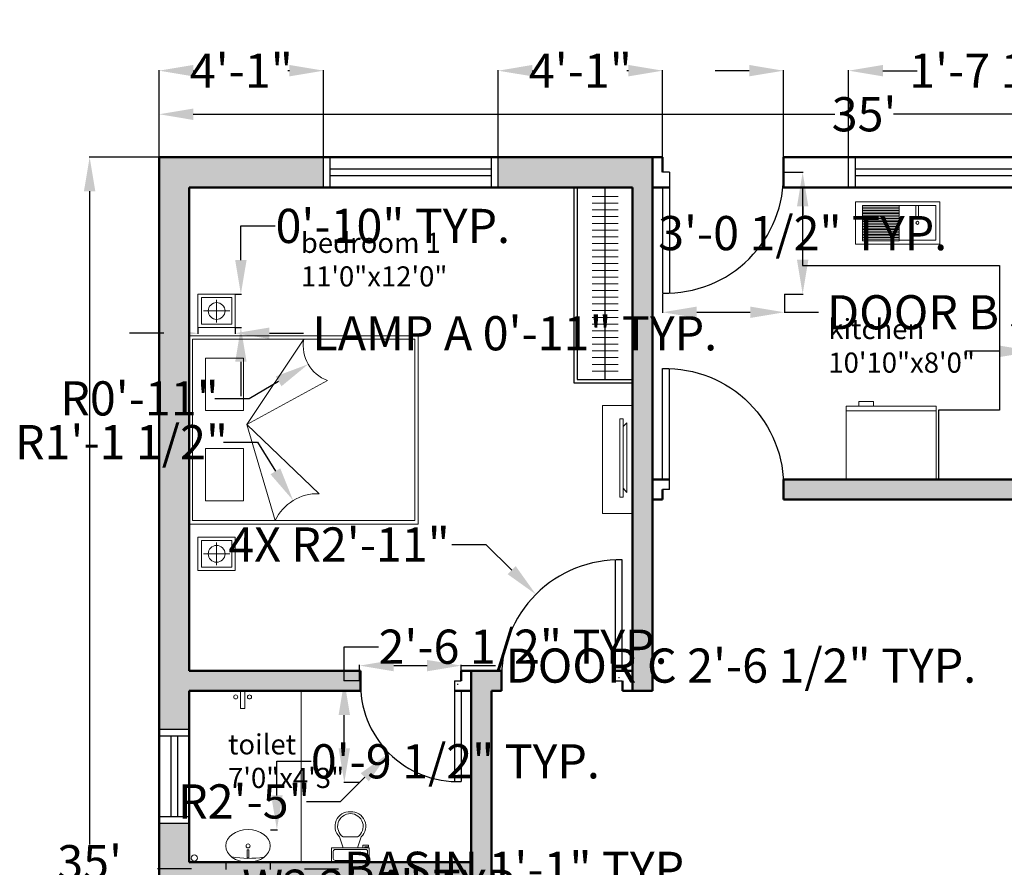
# Model space of a CAD drawing. Units: inches. Extents: x 18 to 9768, y 4 to 3529.
# Tile 2 of 6: x 8712 to 9006, y 3276 to 3529. Entities that reach past the tile are written whole.
import ezdxf

# ---------------------------------------------------------------- set-up
doc = ezdxf.new("R2010")
doc.units = ezdxf.units.IN
doc.header["$MEASUREMENT"] = 0
for name, color, linetype, lineweight in [('A-ANNO-DIMS', 2, 'Continuous', 18), ('A-AREA-IDEN', 7, 'Continuous', 18), ('A-CASE-PATT', 9, 'Continuous', 13), ('A-EQPM', 8, 'Continuous', 18), ('A-FLOR-CASE', 9, 'Continuous', 25), ('A-FLOR-FIXT', 9, 'Continuous', 18), ('A-FURN', 8, 'Continuous', 18), ('A-WALL-PATT', 252, 'Continuous', 13), ('WAL', 7, 'Continuous', 50)]:
    doc.layers.add(name, color=color, linetype=linetype, lineweight=lineweight)
doc.layers.add('A-DOOR', color=30, linetype='Continuous', lineweight=25, true_color=0xf8991e)
doc.layers.add('A-GLAZ', color=177, linetype='Continuous', lineweight=25, true_color=0x293189)
doc.styles.get("Standard").update_dxf_attribs({"font": 'arial.ttf'})
doc.dimstyles.get("Standard").update_dxf_attribs({"dimtxt": 10.18, "dimasz": 10.18, "dimexe": 0.18, "dimexo": 0.0625, "dimgap": 0.09, "dimtad": 0, "dimtih": 1, "dimtoh": 1, "dimdec": 0, "dimzin": 0, "dimdsep": 46, "dimlunit": 3, "dimtxsty": 'Standard', "dimcen": 0.09, "dimadec": 0, "dimazin": 0, "dimtfac": 1, "dimtdec": 0, "dimtofl": 0, "dimtmove": 0, "dimatfit": 3, "dimfxl": 1, "dimtolj": 1, "dimtzin": 0, "dimarcsym": 0})

# ---------------------------------------------------------------- blocks, each defined once
blk = doc.blocks.new('*U2')
for p, q in [((9.5, -6), (9.5, -2)), ((-10, -8.5), (-8, -8.5)), ((-10, -9.5), (-10, -8.5)), ((-7, -9.5), (-10, -9.5)), ((-8, -8.5), (-8, -8)), ((-7, -8), (-7, -9.5)), ((-4, -8), (-6, -14)), ((4, -8), (6, -14)), ((4, -14), (-4, -14))]:
    blk.add_line(p, q)
blk.add_lwpolyline([(10.5, -8), (10.5, 0), (-10.5, 0), (-10.5, -8)], close=True)
for points in [[(-9.5, -2), (-9.5, -6)], [(8.5, -1), (-8.5, -1)], [(-8.5, -7), (8.5, -7)]]:
    blk.add_lwpolyline(points)
for centre, radius, start, end in [((-8.625, -1.875), 0.8839, 81.8699, 188.1301), ((8.625, -1.875), 0.8839, 351.8699, 98.1301), ((-8.625, -6.125), 0.8839, 171.869898, 278.1301), ((8.625, -6.125), 0.8839, 261.8699, 8.1301), ((-0.4772, -19.9188), 8.0953, 133.01722, 273.38), ((0.0374, -19.8731), 7.127, 124.50543, 269.7), ((-0.0373, -19.8731), 7.127, 270.3, 55.4946), ((0.4773, -19.9188), 8.0953, 266.62, 46.9828)]:
    blk.add_arc(centre, radius, start, end)
blk = doc.blocks.new('*D3')
at = {"layer": 'A-ANNO-DIMS', "color": 0, "lineweight": -2, "transparency": 16777216}
for p, q in [((8753.89, 3487.8), (8753.89, 3500.68)), ((8764.07, 3500.5), (8955.16, 3500.5)), ((9163.71, 3500.5), (8972.61, 3500.5)), ((9173.89, 3487.8), (9173.89, 3500.68))]:
    blk.add_line(p, q, dxfattribs=at)
at = {"layer": 'A-ANNO-DIMS', "color": 0, "transparency": 16777216}
for points in [[(8764.07, 3502.19), (8764.07, 3498.8), (8753.89, 3500.5)], [(9163.71, 3502.19), (9163.71, 3498.8), (9173.89, 3500.5)]]:
    blk.add_solid(points, dxfattribs=at)
at = {"layer": 'Defpoints', "color": 0, "transparency": 16777216}
for p in [(9173.89, 3500.5), (8753.89, 3487.73), (9173.89, 3487.73)]:
    blk.add_point(p, dxfattribs=at)
at = {"layer": 'A-ANNO-DIMS', "color": 0, "transparency": 16777216, "insert": (8963.89, 3500.5), "char_height": 10.18, "attachment_point": 5}
blk.add_mtext("\\A1;35'", dxfattribs=at)
blk = doc.blocks.new('*D4')
at = {"layer": 'A-ANNO-DIMS', "color": 0, "lineweight": -2, "transparency": 16777216}
for p, q in [((8753.82, 3487.73), (8733.02, 3487.73)), ((8733.2, 3477.55), (8733.2, 3283.03)), ((8733.2, 3077.91), (8733.2, 3272.44)), ((8753.82, 3067.73), (8733.02, 3067.73))]:
    blk.add_line(p, q, dxfattribs=at)
at = {"layer": 'A-ANNO-DIMS', "color": 0, "transparency": 16777216}
for points in [[(8731.5, 3477.55), (8734.9, 3477.55), (8733.2, 3487.73)], [(8731.5, 3077.91), (8734.9, 3077.91), (8733.2, 3067.73)]]:
    blk.add_solid(points, dxfattribs=at)
at = {"layer": 'Defpoints', "color": 0, "transparency": 16777216}
for p in [(8753.89, 3487.73), (8733.2, 3067.73), (8753.89, 3067.73)]:
    blk.add_point(p, dxfattribs=at)
at = {"layer": 'A-ANNO-DIMS', "color": 0, "transparency": 16777216, "insert": (8733.2, 3277.73), "char_height": 10.18, "attachment_point": 5}
blk.add_mtext("\\A1;35'", dxfattribs=at)
blk = doc.blocks.new('WINDOW-48')
for p, q in [((0, 0), (0, 9)), ((2, 0), (2, 9)), ((50, 0), (50, 9)), ((52, 0), (52, 9)), ((2, 5.5), (50, 5.5)), ((2, 3.5), (50, 3.5))]:
    blk.add_line(p, q)
blk = doc.blocks.new('WINDOW-24')
for p, q in [((9, 28), (0, 28)), ((9, 26), (0, 26)), ((3.5, 26), (3.5, 2)), ((5.5, 26), (5.5, 2)), ((9, 2), (0, 2)), ((9, 0), (0, 0))]:
    blk.add_line(p, q)
blk = doc.blocks.new('DOOR-36-W6')
for p, q in [((34.01, 0), (34.01, 36)), ((36.01, 3), (36.01, 36)), ((34.01, 0), (36.01, 0))]:
    blk.add_line(p, q)
blk.add_arc((35.01, 1), 35.01, 88.3634, 181.6366)
blk = doc.blocks.new('DOOR-36-W9')
for p, q in [((2, 36.01), (0, 36.01)), ((2, 36.01), (2, 0.01)), ((0, 31.51), (0, 0.01))]:
    blk.add_line(p, q)
blk.add_arc((1, 35.01), 35.01, 268.3634, 1.6366)
blk = doc.blocks.new('DOOR-30-W6')
for p, q in [((28.02, 30.02), (28.02, 0.02)), ((28.02, 30.02), (30.02, 30.02)), ((30.02, 27.02), (30.02, 0.02))]:
    blk.add_line(p, q)
blk.add_arc((29.02, 29.02), 29.02, 178.0251, 271.9749)
blk = doc.blocks.new('LAVATORY-OVAL')
for points in [[(6.91, 1.13), (6.91, 3.63), (6.32, 3.63), (6.32, 1.13)], [(6.32, 1.31), (6.32, 1.3), (6.91, 1.3), (6.91, 1.31)]]:
    blk.add_lwpolyline(points)
blk.add_circle((6.62, 4.84), 0.598)
blk.add_arc((6.8, 30.78), 29.65, 260.185, 278.8899)
blk.add_ellipse((6.62, 4.84), major_axis=(6.62, 0), ratio=0.731413)
blk = doc.blocks.new('NIGHTSTAND-LAMP-A')
for p, q in [((5.56, 8.32), (5.56, 1.55)), ((5.55, 4.97), (1.67, 4.97)), ((1.67, 4.97), (9.46, 4.97))]:
    blk.add_line(p, q)
for points in [[(0, 9.94), (11.1, 9.94), (11.1, 0), (0, 0)], [(1, 8.94), (10.1, 8.94), (10.1, 1), (1, 1)]]:
    blk.add_lwpolyline(points, close=True)
blk.add_circle((5.55, 4.97), 2.5)
blk = doc.blocks.new('*D27')
at = {"layer": 'A-ANNO-DIMS', "color": 0, "lineweight": -2, "transparency": 16777216}
for p, q in [((8767.09, 3260.23), (8767.09, 3270.41)), ((8767.09, 3270.41), (8777.27, 3270.41)), ((8762.95, 3260.23), (8767.27, 3260.23)), ((8767.09, 3242.41), (8767.09, 3250.05)), ((8762.95, 3232.23), (8767.27, 3232.23))]:
    blk.add_line(p, q, dxfattribs=at)
at = {"layer": 'A-ANNO-DIMS', "color": 0, "transparency": 16777216}
for points in [[(8765.39, 3250.05), (8768.78, 3250.05), (8767.09, 3260.23)], [(8765.39, 3242.41), (8768.78, 3242.41), (8767.09, 3232.23)]]:
    blk.add_solid(points, dxfattribs=at)
at = {"layer": 'Defpoints', "color": 0, "transparency": 16777216}
for p in [(8762.89, 3260.23), (8767.09, 3260.23), (8762.89, 3232.23)]:
    blk.add_point(p, dxfattribs=at)
at = {"layer": 'A-ANNO-DIMS', "color": 0, "transparency": 16777216, "insert": (8821.23, 3270.41), "char_height": 10.18, "attachment_point": 5}
blk.add_mtext('\\A1;W2 2\'-4" TYP.', dxfattribs=at)
blk = doc.blocks.new('*D31')
at = {"layer": 'A-ANNO-DIMS', "color": 0, "lineweight": -2, "transparency": 16777216}
for p, q in [((8903.89, 3446.9), (8903.89, 3441.34)), ((8940.16, 3446.9), (8940.16, 3441.34)), ((8914.07, 3441.52), (8929.98, 3441.52)), ((8940.16, 3441.52), (8950.34, 3441.52))]:
    blk.add_line(p, q, dxfattribs=at)
at = {"layer": 'A-ANNO-DIMS', "color": 0, "transparency": 16777216}
for points in [[(8914.07, 3443.21), (8914.07, 3439.82), (8903.89, 3441.52)], [(8929.98, 3443.21), (8929.98, 3439.82), (8940.16, 3441.52)]]:
    blk.add_solid(points, dxfattribs=at)
at = {"layer": 'Defpoints', "color": 0, "transparency": 16777216}
for p in [(8903.89, 3446.96), (8940.16, 3446.96), (8940.16, 3441.52)]:
    blk.add_point(p, dxfattribs=at)
at = {"layer": 'A-ANNO-DIMS', "color": 0, "transparency": 16777216, "insert": (9023.09, 3441.52), "char_height": 10.18, "attachment_point": 5}
blk.add_mtext('\\A1;DOOR B 3\'-0 1/2" TYP.', dxfattribs=at)
blk = doc.blocks.new('*D32')
at = {"layer": 'A-ANNO-DIMS', "color": 0, "lineweight": -2, "transparency": 16777216}
for p, q in [((8940.22, 3483.23), (8945.78, 3483.23)), ((8945.6, 3473.05), (8945.6, 3470.45)), ((8945.6, 3457.14), (8945.6, 3459.74)), ((8940.22, 3446.96), (8945.78, 3446.96))]:
    blk.add_line(p, q, dxfattribs=at)
at = {"layer": 'A-ANNO-DIMS', "color": 0, "transparency": 16777216}
for points in [[(8943.9, 3473.05), (8947.3, 3473.05), (8945.6, 3483.23)], [(8943.9, 3457.14), (8947.3, 3457.14), (8945.6, 3446.96)]]:
    blk.add_solid(points, dxfattribs=at)
at = {"layer": 'Defpoints', "color": 0, "transparency": 16777216}
for p in [(8940.16, 3483.23), (8945.6, 3483.23), (8940.16, 3446.96)]:
    blk.add_point(p, dxfattribs=at)
at = {"layer": 'A-ANNO-DIMS', "color": 0, "transparency": 16777216, "insert": (8945.6, 3465.1), "char_height": 10.18, "attachment_point": 5}
blk.add_mtext('\\A1;3\'-0 1/2" TYP.', dxfattribs=at)
blk = doc.blocks.new('*D33')
at = {"layer": 'A-ANNO-DIMS', "color": 0, "lineweight": -2, "transparency": 16777216}
for p, q in [((8813.61, 3331.8), (8813.61, 3336.46)), ((8823.79, 3336.28), (8833.71, 3336.28)), ((8843.89, 3331.8), (8843.89, 3336.46)), ((8843.89, 3336.28), (8854.07, 3336.28))]:
    blk.add_line(p, q, dxfattribs=at)
at = {"layer": 'A-ANNO-DIMS', "color": 0, "transparency": 16777216}
for points in [[(8823.79, 3337.97), (8823.79, 3334.58), (8813.61, 3336.28)], [(8833.71, 3337.97), (8833.71, 3334.58), (8843.89, 3336.28)]]:
    blk.add_solid(points, dxfattribs=at)
at = {"layer": 'Defpoints', "color": 0, "transparency": 16777216}
for p in [(8843.89, 3336.28), (8813.61, 3331.73), (8843.89, 3331.73)]:
    blk.add_point(p, dxfattribs=at)
at = {"layer": 'A-ANNO-DIMS', "color": 0, "transparency": 16777216, "insert": (8927.21, 3336.28), "char_height": 10.18, "attachment_point": 5}
blk.add_mtext('\\A1;DOOR C 2\'-6 1/2" TYP.', dxfattribs=at)
blk = doc.blocks.new('*D34')
at = {"layer": 'A-ANNO-DIMS', "color": 0, "lineweight": -2, "transparency": 16777216}
for p, q in [((8809.07, 3331.73), (8809.07, 3341.91)), ((8809.07, 3341.91), (8819.25, 3341.91)), ((8813.55, 3331.73), (8808.89, 3331.73)), ((8809.07, 3311.64), (8809.07, 3321.55)), ((8813.55, 3301.46), (8808.89, 3301.46))]:
    blk.add_line(p, q, dxfattribs=at)
at = {"layer": 'A-ANNO-DIMS', "color": 0, "transparency": 16777216}
for points in [[(8807.37, 3321.55), (8810.76, 3321.55), (8809.07, 3331.73)], [(8807.37, 3311.64), (8810.76, 3311.64), (8809.07, 3301.46)]]:
    blk.add_solid(points, dxfattribs=at)
at = {"layer": 'Defpoints', "color": 0, "transparency": 16777216}
for p in [(8809.07, 3331.73), (8813.61, 3331.73), (8813.61, 3301.46)]:
    blk.add_point(p, dxfattribs=at)
at = {"layer": 'A-ANNO-DIMS', "color": 0, "transparency": 16777216, "insert": (8862.31, 3341.91), "char_height": 10.18, "attachment_point": 5}
blk.add_mtext('\\A1;2\'-6 1/2" TYP.', dxfattribs=at)
blk = doc.blocks.new('*D42')
at = {"layer": 'A-ANNO-DIMS', "color": 0, "lineweight": -2, "transparency": 16777216}
for p, q in [((9004.32, 3429.89), (8994.14, 3429.89)), ((9014.5, 3428.39), (9014.5, 3430.07)), ((9023.29, 3428.39), (9023.29, 3430.07)), ((9033.47, 3429.89), (9043.65, 3429.89))]:
    blk.add_line(p, q, dxfattribs=at)
at = {"layer": 'A-ANNO-DIMS', "color": 0, "transparency": 16777216}
for points in [[(9004.32, 3431.58), (9004.32, 3428.19), (9014.5, 3429.89)], [(9033.47, 3431.58), (9033.47, 3428.19), (9023.29, 3429.89)]]:
    blk.add_solid(points, dxfattribs=at)
at = {"layer": 'Defpoints', "color": 0, "transparency": 16777216}
for p in [(9023.29, 3429.89), (9014.5, 3428.32), (9023.29, 3428.32)]:
    blk.add_point(p, dxfattribs=at)
at = {"layer": 'A-ANNO-DIMS', "color": 0, "transparency": 16777216, "insert": (9074.76, 3429.89), "char_height": 10.18, "attachment_point": 5}
blk.add_mtext('\\A1;0\'-9" TYP.', dxfattribs=at)
blk = doc.blocks.new('*D43')
at = {"layer": 'A-ANNO-DIMS', "color": 0, "lineweight": -2, "transparency": 16777216}
for p, q in [((8773.76, 3277.67), (8773.76, 3275.57)), ((8787, 3277.67), (8787, 3275.57)), ((8763.58, 3275.75), (8753.4, 3275.75)), ((8797.18, 3275.75), (8807.36, 3275.75))]:
    blk.add_line(p, q, dxfattribs=at)
at = {"layer": 'A-ANNO-DIMS', "color": 0, "transparency": 16777216}
for points in [[(8763.58, 3277.45), (8763.58, 3274.05), (8773.76, 3275.75)], [(8797.18, 3277.45), (8797.18, 3274.05), (8787, 3275.75)]]:
    blk.add_solid(points, dxfattribs=at)
at = {"layer": 'Defpoints', "color": 0, "transparency": 16777216}
for p in [(8773.76, 3277.73), (8787, 3277.73), (8787, 3275.75)]:
    blk.add_point(p, dxfattribs=at)
at = {"layer": 'A-ANNO-DIMS', "color": 0, "transparency": 16777216, "insert": (8861.56, 3275.75), "char_height": 10.18, "attachment_point": 5}
blk.add_mtext('\\A1;BASIN 1\'-1" TYP.', dxfattribs=at)
blk = doc.blocks.new('*D44')
at = {"layer": 'A-ANNO-DIMS', "color": 0, "lineweight": -2, "transparency": 16777216}
for p, q in [((8788.98, 3297.59), (8788.98, 3307.77)), ((8788.98, 3307.77), (8799.16, 3307.77)), ((8787.06, 3287.41), (8789.16, 3287.41)), ((8787.06, 3277.73), (8789.16, 3277.73)), ((8788.98, 3267.55), (8788.98, 3257.37))]:
    blk.add_line(p, q, dxfattribs=at)
at = {"layer": 'A-ANNO-DIMS', "color": 0, "transparency": 16777216}
for points in [[(8787.29, 3297.59), (8790.68, 3297.59), (8788.98, 3287.41)], [(8787.29, 3267.55), (8790.68, 3267.55), (8788.98, 3277.73)]]:
    blk.add_solid(points, dxfattribs=at)
at = {"layer": 'Defpoints', "color": 0, "transparency": 16777216}
for p in [(8787, 3287.41), (8788.98, 3287.41), (8787, 3277.73)]:
    blk.add_point(p, dxfattribs=at)
at = {"layer": 'A-ANNO-DIMS', "color": 0, "transparency": 16777216, "insert": (8842.14, 3307.77), "char_height": 10.18, "attachment_point": 5}
blk.add_mtext('\\A1;0\'-9 1/2" TYP.', dxfattribs=at)
blk = doc.blocks.new('*D47')
at = {"layer": 'A-ANNO-DIMS', "color": 0, "lineweight": -2, "transparency": 16777216}
for p, q in [((8755.3, 3435.27), (8745.12, 3435.27)), ((8765.48, 3436.88), (8765.48, 3435.09)), ((8776.59, 3436.88), (8776.59, 3435.09)), ((8786.77, 3435.27), (8796.95, 3435.27))]:
    blk.add_line(p, q, dxfattribs=at)
at = {"layer": 'A-ANNO-DIMS', "color": 0, "transparency": 16777216}
for points in [[(8755.3, 3436.97), (8755.3, 3433.58), (8765.48, 3435.27)], [(8786.77, 3436.97), (8786.77, 3433.58), (8776.59, 3435.27)]]:
    blk.add_solid(points, dxfattribs=at)
at = {"layer": 'Defpoints', "color": 0, "transparency": 16777216}
for p in [(8765.48, 3436.94), (8776.59, 3436.94), (8776.59, 3435.27)]:
    blk.add_point(p, dxfattribs=at)
at = {"layer": 'A-ANNO-DIMS', "color": 0, "transparency": 16777216, "insert": (8859.85, 3435.27), "char_height": 10.18, "attachment_point": 5}
blk.add_mtext('\\A1;LAMP A 0\'-11" TYP.', dxfattribs=at)
blk = doc.blocks.new('*D48')
at = {"layer": 'A-ANNO-DIMS', "color": 0, "lineweight": -2, "transparency": 16777216}
for p, q in [((8778.25, 3457.06), (8778.25, 3467.24)), ((8778.25, 3467.24), (8788.43, 3467.24)), ((8776.65, 3446.88), (8778.43, 3446.88)), ((8776.65, 3436.94), (8778.43, 3436.94)), ((8778.25, 3426.76), (8778.25, 3416.58))]:
    blk.add_line(p, q, dxfattribs=at)
at = {"layer": 'A-ANNO-DIMS', "color": 0, "transparency": 16777216}
for points in [[(8776.56, 3457.06), (8779.95, 3457.06), (8778.25, 3446.88)], [(8776.56, 3426.76), (8779.95, 3426.76), (8778.25, 3436.94)]]:
    blk.add_solid(points, dxfattribs=at)
at = {"layer": 'Defpoints', "color": 0, "transparency": 16777216}
for p in [(8776.59, 3446.88), (8778.25, 3446.88), (8776.59, 3436.94)]:
    blk.add_point(p, dxfattribs=at)
at = {"layer": 'A-ANNO-DIMS', "color": 0, "transparency": 16777216, "insert": (8823.51, 3467.24), "char_height": 10.18, "attachment_point": 5}
blk.add_mtext('\\A1;0\'-10" TYP.', dxfattribs=at)
blk = doc.blocks.new('*D68')
at = {"layer": 'A-ANNO-DIMS', "color": 0, "lineweight": -2, "transparency": 16777216}
for p, q in [((8753.89, 3487.8), (8753.89, 3513.66)), ((8764.07, 3513.48), (8764.56, 3513.48)), ((8792.71, 3513.48), (8792.21, 3513.48)), ((8802.89, 3487.8), (8802.89, 3513.66))]:
    blk.add_line(p, q, dxfattribs=at)
at = {"layer": 'A-ANNO-DIMS', "color": 0, "transparency": 16777216}
for points in [[(8764.07, 3515.18), (8764.07, 3511.79), (8753.89, 3513.48)], [(8792.71, 3515.18), (8792.71, 3511.79), (8802.89, 3513.48)]]:
    blk.add_solid(points, dxfattribs=at)
at = {"layer": 'Defpoints', "color": 0, "transparency": 16777216}
for p in [(8802.89, 3513.48), (8753.89, 3487.73), (8802.89, 3487.73)]:
    blk.add_point(p, dxfattribs=at)
at = {"layer": 'A-ANNO-DIMS', "color": 0, "transparency": 16777216, "insert": (8778.39, 3513.48), "char_height": 10.18, "attachment_point": 5}
blk.add_mtext('\\A1;4\'-1"', dxfattribs=at)
blk = doc.blocks.new('*D69')
at = {"layer": 'A-ANNO-DIMS', "color": 0, "lineweight": -2, "transparency": 16777216}
for p, q in [((8854.89, 3487.8), (8854.89, 3513.66)), ((8865.07, 3513.48), (8865.56, 3513.48)), ((8893.71, 3513.48), (8893.21, 3513.48)), ((8903.89, 3487.8), (8903.89, 3513.66))]:
    blk.add_line(p, q, dxfattribs=at)
at = {"layer": 'A-ANNO-DIMS', "color": 0, "transparency": 16777216}
for points in [[(8865.07, 3515.18), (8865.07, 3511.79), (8854.89, 3513.48)], [(8893.71, 3515.18), (8893.71, 3511.79), (8903.89, 3513.48)]]:
    blk.add_solid(points, dxfattribs=at)
at = {"layer": 'Defpoints', "color": 0, "transparency": 16777216}
for p in [(8903.89, 3513.48), (8854.89, 3487.73), (8903.89, 3487.73)]:
    blk.add_point(p, dxfattribs=at)
at = {"layer": 'A-ANNO-DIMS', "color": 0, "transparency": 16777216, "insert": (8879.39, 3513.48), "char_height": 10.18, "attachment_point": 5}
blk.add_mtext('\\A1;4\'-1"', dxfattribs=at)
blk = doc.blocks.new('*D70')
at = {"layer": 'A-ANNO-DIMS', "color": 0, "lineweight": -2, "transparency": 16777216}
for p, q in [((8929.71, 3513.48), (8919.53, 3513.48)), ((8939.89, 3487.8), (8939.89, 3513.66)), ((8959.3, 3487.8), (8959.3, 3513.66)), ((8969.48, 3513.48), (8979.66, 3513.48))]:
    blk.add_line(p, q, dxfattribs=at)
at = {"layer": 'A-ANNO-DIMS', "color": 0, "transparency": 16777216}
for points in [[(8929.71, 3515.18), (8929.71, 3511.79), (8939.89, 3513.48)], [(8969.48, 3515.18), (8969.48, 3511.79), (8959.3, 3513.48)]]:
    blk.add_solid(points, dxfattribs=at)
at = {"layer": 'Defpoints', "color": 0, "transparency": 16777216}
for p in [(8959.3, 3513.48), (8939.89, 3487.73), (8959.3, 3487.73)]:
    blk.add_point(p, dxfattribs=at)
at = {"layer": 'A-ANNO-DIMS', "color": 0, "transparency": 16777216, "insert": (9004.67, 3513.48), "char_height": 10.18, "attachment_point": 5}
blk.add_mtext('\\A1;1\'-7 1/2"', dxfattribs=at)
blk = doc.blocks.new('*D81')
at = {"layer": 'A-ANNO-DIMS', "color": 0, "lineweight": -2, "transparency": 16777216}
for p, q in [((8841.09, 3372.35), (8851.27, 3372.35)), ((8851.27, 3372.35), (8858.93, 3364.69)), ((8890.8, 3332.73), (8890.98, 3332.73)), ((8890.89, 3332.64), (8890.89, 3332.82))]:
    blk.add_line(p, q, dxfattribs=at)
at = {"layer": 'A-ANNO-DIMS', "color": 0, "transparency": 16777216}
blk.add_solid([(8860.13, 3365.89), (8857.73, 3363.49), (8866.13, 3357.49)], dxfattribs=at)
at = {"layer": 'Defpoints', "color": 0, "transparency": 16777216}
for p in [(8866.13, 3357.49), (8890.89, 3332.73)]:
    blk.add_point(p, dxfattribs=at)
at = {"layer": 'A-ANNO-DIMS', "color": 0, "transparency": 16777216, "insert": (8807.5, 3372.35), "char_height": 10.18, "attachment_point": 5}
blk.add_mtext('\\A1;4X R2\'-11"', dxfattribs=at)
blk = doc.blocks.new('*D86')
at = {"layer": 'A-ANNO-DIMS', "color": 0, "lineweight": -2, "transparency": 16777216}
for p, q in [((8842.8, 3330.73), (8842.98, 3330.73)), ((8842.89, 3330.64), (8842.89, 3330.82)), ((8807.97, 3295.82), (8815.17, 3303.02)), ((8797.79, 3295.82), (8807.97, 3295.82))]:
    blk.add_line(p, q, dxfattribs=at)
at = {"layer": 'A-ANNO-DIMS', "color": 0, "transparency": 16777216}
blk.add_solid([(8813.97, 3304.22), (8816.37, 3301.82), (8822.37, 3310.22)], dxfattribs=at)
at = {"layer": 'Defpoints', "color": 0, "transparency": 16777216}
for p in [(8842.89, 3330.73), (8822.37, 3310.22)]:
    blk.add_point(p, dxfattribs=at)
at = {"layer": 'A-ANNO-DIMS', "color": 0, "transparency": 16777216, "insert": (8779.3, 3295.82), "char_height": 10.18, "attachment_point": 5}
blk.add_mtext('\\A1;R2\'-5"', dxfattribs=at)
blk = doc.blocks.new('*D88')
at = {"layer": 'A-ANNO-DIMS', "color": 0, "lineweight": -2, "transparency": 16777216}
for p, q in [((8773.05, 3402.84), (8783.23, 3402.84)), ((8783.23, 3402.84), (8788.53, 3394.15)), ((8800.89, 3373.73), (8801.07, 3373.73)), ((8800.98, 3373.64), (8800.98, 3373.82))]:
    blk.add_line(p, q, dxfattribs=at)
at = {"layer": 'A-ANNO-DIMS', "color": 0, "transparency": 16777216}
blk.add_solid([(8789.98, 3395.03), (8787.08, 3393.27), (8793.83, 3385.46)], dxfattribs=at)
at = {"layer": 'Defpoints', "color": 0, "transparency": 16777216}
for p in [(8793.83, 3385.46), (8800.98, 3373.73)]:
    blk.add_point(p, dxfattribs=at)
at = {"layer": 'A-ANNO-DIMS', "color": 0, "transparency": 16777216, "insert": (8742.7, 3402.84), "char_height": 10.18, "attachment_point": 5}
blk.add_mtext('\\A1;R1\'-1 1/2"', dxfattribs=at)
blk = doc.blocks.new('*D89')
at = {"layer": 'A-ANNO-DIMS', "color": 0, "lineweight": -2, "transparency": 16777216}
for p, q in [((8807.89, 3431.63), (8808.07, 3431.63)), ((8807.98, 3431.54), (8807.98, 3431.72)), ((8780.68, 3415.87), (8789.5, 3420.96)), ((8770.5, 3415.87), (8780.68, 3415.87))]:
    blk.add_line(p, q, dxfattribs=at)
at = {"layer": 'A-ANNO-DIMS', "color": 0, "transparency": 16777216}
blk.add_solid([(8788.65, 3422.43), (8790.35, 3419.49), (8798.31, 3426.05)], dxfattribs=at)
at = {"layer": 'Defpoints', "color": 0, "transparency": 16777216}
for p in [(8807.98, 3431.63), (8798.31, 3426.05)]:
    blk.add_point(p, dxfattribs=at)
at = {"layer": 'A-ANNO-DIMS', "color": 0, "transparency": 16777216, "insert": (8748.06, 3415.87), "char_height": 10.18, "attachment_point": 5}
blk.add_mtext('\\A1;R0\'-11"', dxfattribs=at)

msp = doc.modelspace()

# ---------------------------------------------------------------- hatches: boundary and pattern name
at = {"layer": 'A-CASE-PATT'}
h = msp.add_hatch(dxfattribs=at)
h.set_pattern_fill('ANSI31', color=256, scale=16, angle=-45, style=0)
h.paths.add_polyline_path([(8882.88, 3422.9), (8890.67, 3422.9), (8890.67, 3476.9), (8882.88, 3476.9)])
at = {"layer": 'A-WALL-PATT'}
h = msp.add_hatch(color=256, dxfattribs=at)
h.dxf.hatch_style = 1
h.paths.add_polyline_path([(8762.89, 3478.73), (8802.89, 3478.73), (8802.89, 3487.73), (8753.89, 3487.73), (8753.89, 3317.23), (8762.89, 3317.23), (8762.89, 3328.73), (8813.89, 3328.73), (8813.89, 3329.73, -0.017236), (8813.89, 3331.73), (8813.89, 3334.73), (8762.89, 3334.73)])
h.paths.add_polyline_path([(8900.89, 3487.73), (8854.89, 3487.73), (8854.89, 3478.73), (8894.89, 3478.73), (8894.89, 3421.46), (8894.89, 3334.73), (8894.89, 3328.73), (8900.89, 3328.73), (8900.89, 3391.73), (8900.89, 3478.73)])
h.paths.add_polyline_path([(9074.89, 3487.73), (9011.3, 3487.73), (9011.3, 3478.73), (9030.89, 3478.73), (9030.89, 3391.73), (8939.89, 3391.73), (8939.89, 3390.73, -0.014283), (8939.89, 3388.73), (8939.89, 3385.73), (9030.89, 3385.73), (9030.89, 3373.73), (9033.89, 3373.73, -0.014283), (9035.89, 3373.73), (9036.89, 3373.73), (9036.89, 3478.73), (9074.89, 3478.73)])
h.paths.add_polyline_path([(9173.89, 3487.73), (9126.89, 3487.73), (9126.89, 3478.73), (9128.34, 3478.73), (9164.89, 3478.73), (9164.89, 3334.73), (9147.51, 3334.73), (9036.89, 3334.73), (9030.89, 3334.73), (9030.89, 3328.73), (9164.89, 3328.73), (9164.89, 3300.73), (9173.89, 3300.73)])
h.paths.add_polyline_path([(8762.89, 3271.73), (8846.89, 3271.73), (8852.89, 3271.73), (8852.89, 3328.73), (8855.89, 3328.73), (8855.89, 3331.73, -0.014283), (8855.89, 3333.73), (8855.89, 3334.73), (8846.89, 3334.73), (8846.89, 3328.73), (8846.89, 3277.73), (8762.89, 3277.73), (8762.89, 3289.23), (8753.89, 3289.23), (8753.89, 3260.23), (8762.89, 3260.23)])
h.paths.add_polyline_path([(8762.89, 3214.73), (8855.89, 3214.73), (8855.89, 3215.73, -0.014283), (8855.89, 3217.73), (8855.89, 3220.73), (8852.89, 3220.73), (8852.89, 3238.73), (8849.89, 3238.73, -0.017236), (8847.89, 3238.73), (8846.89, 3238.73), (8846.89, 3220.73), (8762.89, 3220.73), (8762.89, 3232.23), (8753.89, 3232.23), (8753.89, 3171.73), (8762.89, 3171.73)])
h.paths.add_polyline_path([(8762.89, 3119.73), (8753.89, 3119.73), (8753.89, 3067.73), (8802.89, 3067.73), (8802.89, 3076.73), (8795.03, 3076.73), (8762.89, 3076.73)])
h.paths.add_polyline_path([(8900.89, 3076.73), (8900.89, 3214.73), (8987.37, 3214.73), (8987.37, 3220.73), (8894.89, 3220.73), (8894.89, 3214.73), (8894.89, 3076.73), (8854.89, 3076.73), (8854.89, 3067.73), (8900.89, 3067.73)])
h.paths.add_polyline_path([(9074.89, 3076.73), (9071.87, 3076.73), (9036.89, 3076.73), (9036.89, 3214.73), (9036.89, 3220.73), (9030.89, 3220.73), (9030.89, 3214.73), (9030.89, 3076.73), (9030.89, 3067.73), (9074.89, 3067.73)])
h.paths.add_polyline_path([(9173.89, 3119.73), (9164.89, 3119.73), (9164.89, 3076.73), (9126.89, 3076.73), (9126.89, 3067.73), (9173.89, 3067.73)])
h.paths.add_polyline_path([(9173.89, 3248.73), (9164.89, 3248.73), (9164.89, 3220.73), (9075.89, 3220.73), (9075.89, 3217.73, -0.014283), (9075.89, 3215.73), (9075.89, 3214.73), (9164.89, 3214.73), (9164.89, 3171.73), (9173.89, 3171.73)])

# ---------------------------------------------------------------- linework, layer by layer
at = {"layer": 'A-EQPM'}
for p, q in [((8958.53, 3412.16), (8985.36, 3412.16)), ((8892.11, 3407.5), (8893.24, 3408.59)), ((8893.24, 3408.59), (8893.24, 3387.83)), ((8893.24, 3387.83), (8892.11, 3389.09))]:
    msp.add_line(p, q, dxfattribs=at)
for points in [[(8962.32, 3413.57), (8966.72, 3413.57), (8966.72, 3414.95), (8962.32, 3414.95)], [(8894.89, 3413.78), (8886.02, 3413.78), (8886.02, 3381.54), (8894.89, 3381.54)], [(8985.36, 3391.73), (8958.53, 3391.73), (8958.53, 3413.57), (8985.36, 3413.57)], [(8892.11, 3409.76), (8891.13, 3409.76), (8891.13, 3386.48), (8892.11, 3386.48)]]:
    msp.add_lwpolyline(points, close=True, dxfattribs=at)
at = {"layer": 'A-FLOR-CASE'}
for p, q in [((8886.66, 3478.73), (8886.66, 3421.46)), ((8945.52, 3478.73), (8945.52, 3455.48)), ((8945.52, 3455.48), (9004.2, 3455.48)), ((9004.2, 3455.48), (9004.2, 3412.36)), ((9004.2, 3412.36), (8986.09, 3412.36)), ((8986.09, 3412.36), (8986.09, 3391.73))]:
    msp.add_line(p, q, dxfattribs=at)
msp.add_lwpolyline([(8877.44, 3478.73), (8877.44, 3420.46), (8894.89, 3420.46)], dxfattribs=at)
msp.add_lwpolyline([(8894.89, 3478.73), (8878.44, 3478.73), (8878.44, 3421.46), (8894.89, 3421.46)], close=True, dxfattribs=at)
at = {"layer": 'A-FLOR-FIXT'}
msp.add_line((8796.24, 3328.73), (8796.24, 3277.73), dxfattribs=at)
for points in [[(8961.38, 3474.44), (8986.48, 3474.44), (8986.48, 3461.79), (8961.38, 3461.79)], [(8963.39, 3473.29), (8974.35, 3473.29), (8974.35, 3472.81), (8963.39, 3472.81)], [(8963.39, 3472.81), (8974.35, 3472.81), (8974.35, 3472.33), (8963.39, 3472.33)], [(8985.22, 3473.29), (8974.35, 3473.29), (8974.35, 3463.01), (8985.22, 3463.01)], [(8980.15, 3473.29), (8979.32, 3473.29), (8979.32, 3469.91), (8980.15, 3469.91)], [(8963.39, 3472.33), (8974.35, 3472.33), (8974.35, 3471.86), (8963.39, 3471.86)], [(8963.39, 3471.86), (8974.35, 3471.86), (8974.35, 3471.38), (8963.39, 3471.38)], [(8963.39, 3471.38), (8974.35, 3471.38), (8974.35, 3470.9), (8963.39, 3470.9)], [(8963.39, 3470.9), (8974.35, 3470.9), (8974.35, 3470.43), (8963.39, 3470.43)], [(8963.39, 3470.43), (8974.35, 3470.43), (8974.35, 3469.95), (8963.39, 3469.95)], [(8963.39, 3469.95), (8974.35, 3469.95), (8974.35, 3469.48), (8963.39, 3469.48)], [(8963.39, 3469.48), (8974.35, 3469.48), (8974.35, 3469), (8963.39, 3469)], [(8963.39, 3469), (8974.35, 3469), (8974.35, 3468.52), (8963.39, 3468.52)], [(8963.39, 3468.52), (8974.35, 3468.52), (8974.35, 3468.05), (8963.39, 3468.05)], [(8963.39, 3468.05), (8974.35, 3468.05), (8974.35, 3467.57), (8963.39, 3467.57)], [(8963.39, 3467.57), (8974.35, 3467.57), (8974.35, 3467.09), (8963.39, 3467.09)], [(8963.39, 3467.09), (8974.35, 3467.09), (8974.35, 3466.62), (8963.39, 3466.62)], [(8963.39, 3466.62), (8974.35, 3466.62), (8974.35, 3466.14), (8963.39, 3466.14)], [(8963.39, 3466.14), (8974.35, 3466.14), (8974.35, 3465.66), (8963.39, 3465.66)], [(8963.39, 3465.66), (8974.35, 3465.66), (8974.35, 3465.19), (8963.39, 3465.19)], [(8963.39, 3465.19), (8974.35, 3465.19), (8974.35, 3464.71), (8963.39, 3464.71)], [(8963.39, 3464.71), (8974.35, 3464.71), (8974.35, 3464.24), (8963.39, 3464.24)], [(8963.39, 3464.24), (8974.35, 3464.24), (8974.35, 3463.76), (8963.39, 3463.76)], [(8963.39, 3463.76), (8974.35, 3463.76), (8974.35, 3463.28), (8963.39, 3463.28)], [(8963.39, 3463.28), (8974.35, 3463.28), (8974.35, 3462.81), (8963.39, 3462.81)], [(8779.45, 3328.73), (8778.16, 3328.73), (8778.16, 3323.46), (8779.45, 3323.46)]]:
    msp.add_lwpolyline(points, close=True, dxfattribs=at)
for centre, radius in [((8979.79, 3468.15), 0.462), ((8776.72, 3326.95), 0.609), ((8780.83, 3326.95), 0.609), ((8764.4, 3278.96), 0.909)]:
    msp.add_circle(centre, radius, dxfattribs=at)
at = {"layer": 'A-FURN'}
for p, q in [((8780.04, 3408.13), (8796.97, 3433.46)), ((8804.06, 3421.18), (8780.04, 3408.13)), ((8780.04, 3408.13), (8801.62, 3387.45)), ((8788.49, 3379.45), (8780.04, 3408.13))]:
    msp.add_line(p, q, dxfattribs=at)
for points in [[(8762.89, 3434.46), (8831.06, 3434.46), (8831.06, 3378.45), (8762.89, 3378.45)], [(8763.89, 3433.46), (8830.06, 3433.46), (8830.06, 3379.45), (8763.89, 3379.45)], [(8767.74, 3427.89), (8779.04, 3427.89), (8779.04, 3412.26), (8767.74, 3412.26)], [(8767.74, 3400.97), (8779.04, 3400.97), (8779.04, 3385.34), (8767.74, 3385.34)]]:
    msp.add_lwpolyline(points, close=True, dxfattribs=at)
for centre, radius, start, end in [((8807.98, 3431.63), 11.16, 170.5496, 249.4504), ((8800.98, 3373.73), 13.74, 87.3639, 155.3833)]:
    msp.add_arc(centre, radius, start, end, dxfattribs=at)
at = {"layer": 'WAL'}
for p, q in [((8753.89, 3067.73), (8753.89, 3487.73)), ((8753.89, 3487.73), (8903.89, 3487.73)), ((8900.89, 3478.73), (8900.89, 3487.73)), ((8903.89, 3483.23), (8903.89, 3487.73)), ((8939.89, 3478.73), (8939.89, 3487.73)), ((8939.89, 3487.73), (9173.89, 3487.73)), ((8762.89, 3478.73), (8894.89, 3478.73)), ((8762.89, 3334.73), (8762.89, 3478.73)), ((8894.89, 3334.73), (8894.89, 3478.73)), ((8900.89, 3391.73), (8900.89, 3478.73)), ((8900.89, 3478.73), (8905.89, 3478.73)), ((8939.72, 3478.73), (9030.89, 3478.73)), ((8900.89, 3391.73), (8905.89, 3391.73)), ((8900.89, 3328.73), (8900.89, 3391.73)), ((8939.84, 3391.73), (9030.89, 3391.73)), ((8939.89, 3385.73), (8939.89, 3391.73)), ((8903.89, 3385.73), (8903.89, 3388.73)), ((8900.89, 3385.73), (8903.89, 3385.73)), ((8939.89, 3385.73), (9030.89, 3385.73)), ((8762.89, 3334.73), (8813.89, 3334.73)), ((8813.89, 3328.73), (8813.89, 3334.73)), ((8843.89, 3331.73), (8843.89, 3334.73)), ((8843.89, 3334.73), (8855.93, 3334.73)), ((8846.89, 3328.73), (8846.89, 3334.73)), ((8855.89, 3334.73), (8855.89, 3328.73)), ((8889.89, 3334.73), (8894.89, 3334.73)), ((8894.89, 3334.73), (8894.89, 3328.73)), ((8891.89, 3331.73), (8891.89, 3328.73)), ((8762.89, 3328.73), (8813.94, 3328.73)), ((8762.89, 3277.73), (8762.89, 3328.73)), ((8841.89, 3328.73), (8846.89, 3328.73)), ((8846.89, 3277.73), (8846.89, 3328.73)), ((8852.89, 3271.73), (8852.89, 3328.73)), ((8852.89, 3328.73), (8855.89, 3328.73)), ((8891.89, 3328.73), (8900.89, 3328.73)), ((8762.89, 3277.73), (8846.89, 3277.73))]:
    msp.add_line(p, q, dxfattribs=at)

# ---------------------------------------------------------------- block references
at = {"layer": 'A-DOOR'}
for name, p in [('DOOR-36-W9', (8903.89, 3447.22)), ('DOOR-36-W6', (8855.87, 3331.74)), ('DOOR-30-W6', (8813.87, 3301.72))]:
    msp.add_blockref(name, p, dxfattribs=at)
at = {"layer": 'A-DOOR', "extrusion": (0, 0, -1), "zscale": -1}
msp.add_blockref('DOOR-36-W6', (-8939.9, 3388.74), dxfattribs=at)
at = {"layer": 'A-FLOR-FIXT', "xscale": 0.5359950384494228, "yscale": 0.5359950384494228, "zscale": 0.5359950384494228, "rotation": 180}
msp.add_blockref('*U2', (8810.88, 3277.73), dxfattribs=at)
at = {"layer": 'A-FLOR-FIXT'}
msp.add_blockref('LAVATORY-OVAL', (8773.76, 3277.74), dxfattribs=at)
at = {"layer": 'A-FURN'}
for p in [(8765.48, 3436.94), (8765.48, 3364.61)]:
    msp.add_blockref('NIGHTSTAND-LAMP-A', p, dxfattribs=at)
at = {"layer": 'A-GLAZ'}
for name, p in [('WINDOW-48', (8802.89, 3478.74)), ('WINDOW-48', (8959.3, 3478.74)), ('WINDOW-24', (8753.89, 3289.24))]:
    msp.add_blockref(name, p, dxfattribs=at)

# ---------------------------------------------------------------- texts
at = {"layer": 'A-AREA-IDEN', "char_height": 6, "attachment_point": 1}
for s, insert in [('bedroom 1\\P11\'0"x12\'0"', (8796.12, 3465.2)), ('kitchen\\P10\'10"x8\'0"', (8953.26, 3439.53)), ('toilet\\P7\'0"x4\'3"', (8774.44, 3315.83))]:
    msp.add_mtext_dynamic_manual_height_columns(s, width=53.4573, gutter_width=1, heights=[0], dxfattribs=dict(at, insert=insert))

# ---------------------------------------------------------------- dimensions: what is measured, and where the dimension line sits
at = {"layer": 'A-ANNO-DIMS'}
for base, p1, p2, override, picture, middle in [((8959.3, 3513.48), (8939.89, 3487.73), (8959.3, 3487.73), {"dimdec": 1, "dimlfac": 1, "dimrnd": 0, "dimzin": 1, "dimdsep": 46, "dimlunit": 4, "dimfrac": 2}, '*D70', (9004.67, 3513.48)), ((8802.89, 3513.48), (8753.89, 3487.73), (8802.89, 3487.73), {"dimdec": 1, "dimlfac": 1, "dimrnd": 0, "dimzin": 1, "dimdsep": 46, "dimlunit": 4, "dimfrac": 2}, '*D68', (8778.39, 3513.48)), ((8903.89, 3513.48), (8854.89, 3487.73), (8903.89, 3487.73), {"dimdec": 1, "dimlfac": 1, "dimrnd": 0, "dimzin": 1, "dimdsep": 46, "dimlunit": 4, "dimfrac": 2}, '*D69', (8879.39, 3513.48)), ((9173.89, 3500.5), (8753.89, 3487.73), (9173.89, 3487.73), {"dimclrd": 0, "dimclre": 0, "dimclrt": 0}, '*D3', (8963.89, 3500.5))]:
    dim = msp.add_linear_dim(base=base, p1=p1, p2=p2, dimstyle='Standard', override=override, dxfattribs=at)
    dim.commit()
    dim.dimension.update_dxf_attribs({"geometry": picture, "text_midpoint": middle})
dim = msp.add_linear_dim(base=(8733.2, 3067.73), p1=(8753.89, 3487.73), p2=(8753.89, 3067.73), angle=90, dimstyle='Standard', override={"dimclrd": 0, "dimclre": 0, "dimclrt": 0}, dxfattribs=at)
dim.commit()
dim.dimension.update_dxf_attribs({"geometry": '*D4', "text_midpoint": (8733.2, 3277.73)})
for base, p1, p2, text, picture, middle in [((8945.6, 3483.23), (8940.16, 3446.96), (8940.16, 3483.23), '<> TYP.', '*D32', (8945.6, 3465.1)), ((8778.25, 3446.88), (8776.59, 3436.94), (8776.59, 3446.88), '<> TYP.', '*D48', (8823.51, 3467.24)), ((8809.07, 3331.73), (8813.61, 3301.46), (8813.61, 3331.73), '<> TYP.', '*D34', (8862.31, 3341.91)), ((8788.98, 3287.41), (8787, 3277.73), (8787, 3287.41), '<> TYP.', '*D44', (8842.14, 3307.77)), ((8767.09, 3260.23), (8762.89, 3232.23), (8762.89, 3260.23), 'W2 <> TYP.', '*D27', (8821.23, 3270.41))]:
    dim = msp.add_linear_dim(base=base, p1=p1, p2=p2, angle=90, text=text, dimstyle='Standard', override={"dimdec": 1, "dimlfac": 1, "dimrnd": 0, "dimzin": 1, "dimdsep": 46, "dimlunit": 4, "dimfrac": 2}, dxfattribs=at)
    dim.commit()
    dim.dimension.update_dxf_attribs({"geometry": picture, "text_midpoint": middle})
for base, p1, p2, text, picture, middle in [((8940.16, 3441.52), (8903.89, 3446.96), (8940.16, 3446.96), 'DOOR B <> TYP.', '*D31', (9023.09, 3441.52)), ((8776.59, 3435.27), (8765.48, 3436.94), (8776.59, 3436.94), 'LAMP A <> TYP.', '*D47', (8859.85, 3435.27)), ((9023.29, 3429.89), (9014.5, 3428.32), (9023.29, 3428.32), '<> TYP.', '*D42', (9074.76, 3429.89)), ((8843.89, 3336.28), (8813.61, 3331.73), (8843.89, 3331.73), 'DOOR C <> TYP.', '*D33', (8927.21, 3336.28)), ((8787, 3275.75), (8773.76, 3277.73), (8787, 3277.73), 'BASIN <> TYP.', '*D43', (8861.56, 3275.75))]:
    dim = msp.add_linear_dim(base=base, p1=p1, p2=p2, text=text, dimstyle='Standard', override={"dimdec": 1, "dimlfac": 1, "dimrnd": 0, "dimzin": 1, "dimdsep": 46, "dimlunit": 4, "dimfrac": 2}, dxfattribs=at)
    dim.commit()
    dim.dimension.update_dxf_attribs({"geometry": picture, "text_midpoint": middle})
for center, mpoint, picture, middle in [((8807.98, 3431.63), (8798.31, 3426.05), '*D89', (8748.06, 3415.87)), ((8800.98, 3373.73), (8793.83, 3385.46), '*D88', (8742.7, 3402.84)), ((8842.89, 3330.73), (8822.37, 3310.22), '*D86', (8779.3, 3295.82))]:
    dim = msp.add_radius_dim(center=center, mpoint=mpoint, dimstyle='Standard', override={"dimdec": 1, "dimlfac": 1, "dimrnd": 0, "dimzin": 1, "dimdsep": 46, "dimlunit": 4, "dimfrac": 2}, dxfattribs=at)
    dim.commit()
    dim.dimension.update_dxf_attribs({"geometry": picture, "text_midpoint": middle})
dim = msp.add_radius_dim(center=(8890.89, 3332.73), mpoint=(8866.13, 3357.49), text='4X <>', dimstyle='Standard', override={"dimdec": 1, "dimlfac": 1, "dimrnd": 0, "dimzin": 1, "dimdsep": 46, "dimlunit": 4, "dimfrac": 2}, dxfattribs=at)
dim.commit()
dim.dimension.update_dxf_attribs({"geometry": '*D81', "text_midpoint": (8807.5, 3372.35), "dimtype": 164})

doc.saveas('drawing.dxf')
